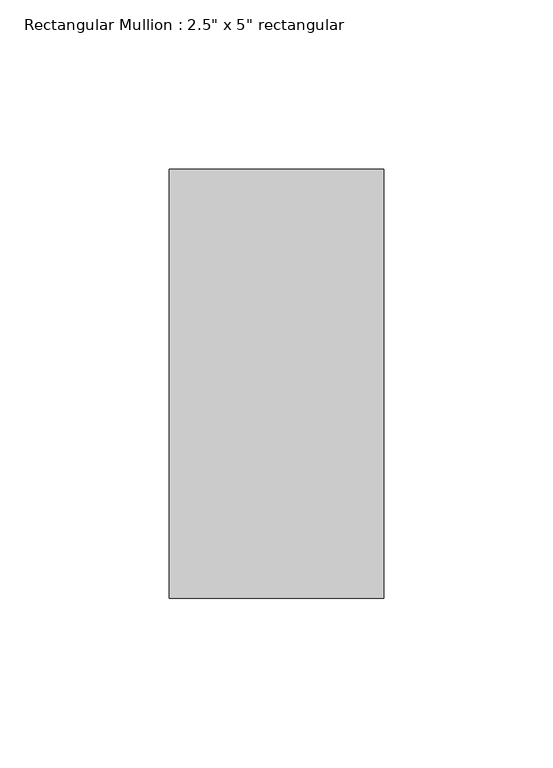
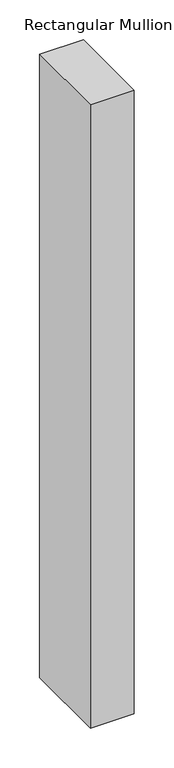
"""IFC4 building model written with IfcOpenShell, lengths in millimetres: member geometry."""

from ifc_helpers import new_model, si_unit, frame, origin, place, context, project, spatial, polyline, outline, extrude, source, transform, mapped, element, save


def member_e1cb8a7d(model_context):
    return source(origin(), model_context, "Body", "SweptSolid", [
        extrude(outline(polyline([(31.75, 63.5), (31.75, -63.5), (-31.75, -63.5), (-31.75, 63.5), (31.75, 63.5)])), frame((0.0, 0.0, -954.428642), z_axis=(0.0, 0.0, 1.0), x_axis=(1.0, 0.0, 0.0)), (0.0, 0.0, 1.0), 954.428642),
    ])


if __name__ == "__main__":
    model = new_model("IFC4")
    model_context = context("Model", 3, world=origin())
    ifc_project = project(units=[si_unit("LENGTHUNIT", "METRE", prefix="MILLI")], contexts=[model_context])
    site = spatial("IfcSite", under=ifc_project)
    building = spatial("IfcBuilding", under=site)
    placement = place(None, origin())
    member_shape = member_e1cb8a7d(model_context)
    element("IfcMember", 1, ObjectType="Rectangular Mullion : 2.5\" x 5\" rectangular", at=placement, inside=building, context=model_context, shape_type="MappedRepresentation", body=[
        mapped(member_shape, transform((0.0, 0.0, 0.0), x_axis=(1.0, 0.0, 0.0), y_axis=(0.0, 1.0, 0.0), z_axis=(0.0, 0.0, 1.0))),
    ])
    save(model, "model.ifc")

# Revit data of these elements
# Type "Rectangular Mullion : 2.5\" x 5\" rectangular"
#   built-in parameter 1007304 = 0.416667 (stored number, unit not read)
#   built-in parameter 1007301 = 0.104167 (stored number, unit not read)
#   built-in parameter 1007300 = 0.104167 (stored number, unit not read)
# Element 1 (IfcMember, "Rectangular Mullion : 2.5\" x 5\" rectangular")
#   Materials on its faces: "Aluminum"
# Materials
#   "Aluminum": class "Metal", colour RGB 247 247 247, transparency 0, Description = "Aluminum 6061", Cost = 0
